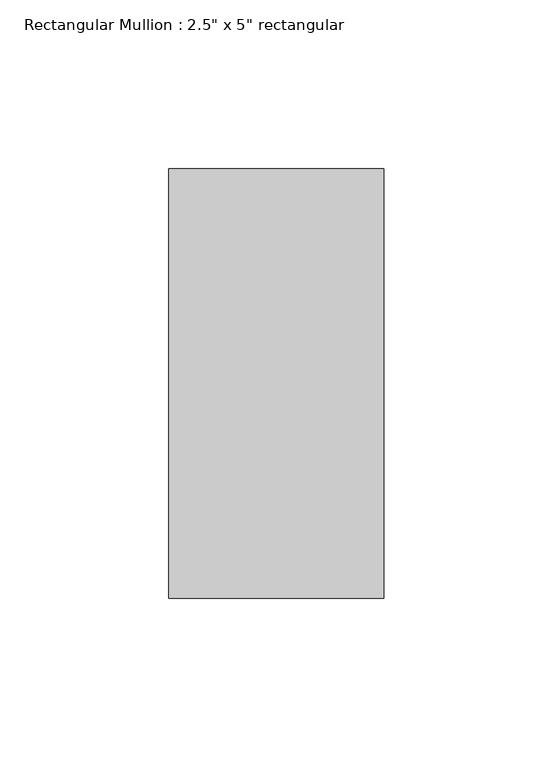
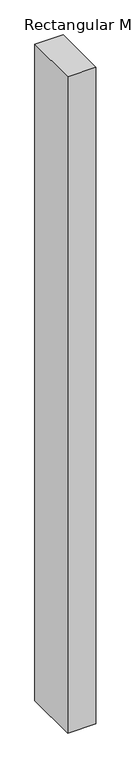
"""IFC4 building model written with IfcOpenShell, lengths in millimetres: member geometry."""

from ifc_helpers import new_model, si_unit, frame, origin, place, context, project, spatial, polyline, outline, extrude, source, transform, mapped, element, save


def member_f05129a9(model_context):
    return source(origin(), model_context, "Body", "SweptSolid", [
        extrude(outline(polyline([(31.75, 63.5), (31.75, -63.5), (-31.75, -63.5), (-31.75, 63.5), (31.75, 63.5)])), frame((0.0, 0.0, -1556.7181357), z_axis=(0.0, 0.0, 1.0), x_axis=(1.0, 0.0, 0.0)), (0.0, 0.0, 1.0), 1556.7181357),
    ])


if __name__ == "__main__":
    model = new_model("IFC4")
    model_context = context("Model", 3, world=origin())
    ifc_project = project(units=[si_unit("LENGTHUNIT", "METRE", prefix="MILLI")], contexts=[model_context])
    site = spatial("IfcSite", under=ifc_project)
    building = spatial("IfcBuilding", under=site)
    placement = place(None, origin())
    member_shape = member_f05129a9(model_context)
    element("IfcMember", 1, ObjectType="Rectangular Mullion : 2.5\" x 5\" rectangular", at=placement, inside=building, context=model_context, shape_type="MappedRepresentation", body=[
        mapped(member_shape, transform((0.0, 0.0, 0.0), x_axis=(1.0, 0.0, 0.0), y_axis=(0.0, 1.0, 0.0), z_axis=(0.0, 0.0, 1.0))),
    ])
    save(model, "model.ifc")

# Revit data of these elements
# Type "Rectangular Mullion : 2.5\" x 5\" rectangular"
#   built-in parameter 1007304 = 0.416667 (stored number, unit not read)
#   built-in parameter 1007301 = 0.104167 (stored number, unit not read)
#   built-in parameter 1007300 = 0.104167 (stored number, unit not read)
# Element 1 (IfcMember, "Rectangular Mullion : 2.5\" x 5\" rectangular")
#   Materials on its faces: "Aluminum"
# Materials
#   "Aluminum": class "Metal", colour RGB 247 247 247, transparency 0, Description = "Aluminum 6061", Cost = 0
